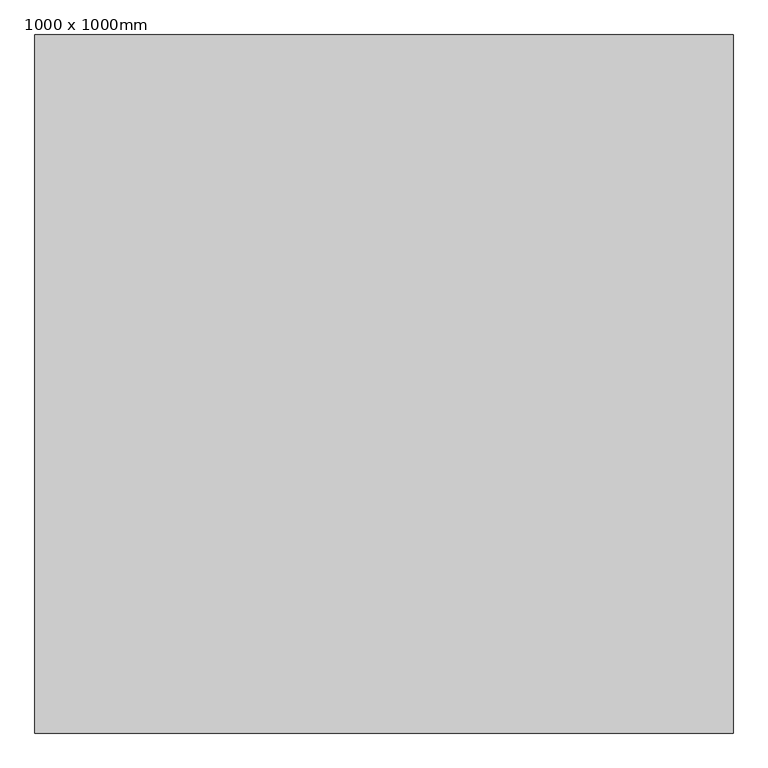
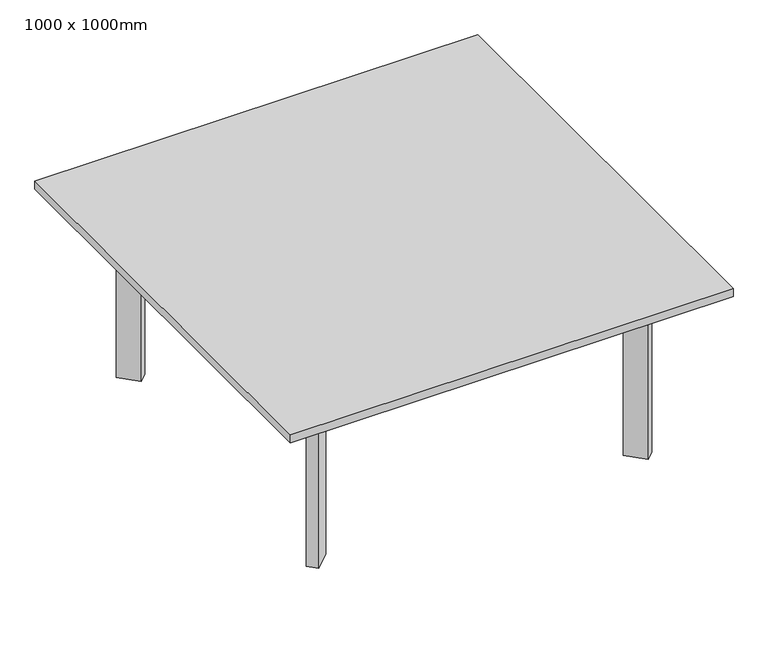
"""IFC4 building model written with IfcOpenShell, lengths in millimetres: furniture geometry, 1000 x 1000mm."""

from ifc_helpers import new_model, si_unit, frame, origin, origin_with_axes, place, context, project, spatial, polyline, outline, extrude, source, transform, mapped, element, save


def furniture_1000_x_1000mm_85c88e14(model_context):
    return source(origin(), model_context, "Body", "SweptSolid", [
        extrude(outline(polyline([(444.6325628, 440.0522349), (444.6325628, -559.9735464), (-555.3932185, -559.9735464), (-555.3932185, 440.0522349), (444.6325628, 440.0522349)])), frame((0.0, 0.0, 410.9640625), z_axis=(0.0, 0.0, 1.0), x_axis=(1.0, 0.0, 0.0)), (0.0, 0.0, 1.0), 19.05),
        extrude(outline(polyline([(-427.4000717, 330.0196004), (-391.4790473, 294.0985759), (-409.4395595, 276.1380637), (-445.360584, 312.0590881), (-427.4000717, 330.0196004)])), origin_with_axes(), (0.0, 0.0, 1.0), 360.1640625),
        extrude(outline(polyline([(316.639416, 330.0196004), (334.5999283, 312.0590881), (298.6789038, 276.1380637), (280.7183915, 294.0985759), (316.639416, 330.0196004)])), origin_with_axes(), (0.0, 0.0, 1.0), 360.1640625),
        extrude(outline(polyline([(334.5999283, -431.9803996), (316.639416, -449.9409119), (280.7183915, -414.0198874), (298.6789038, -396.0593751), (334.5999283, -431.9803996)])), origin_with_axes(), (0.0, 0.0, 1.0), 360.1640625),
        extrude(outline(polyline([(-445.360584, -431.9803996), (-409.4395595, -396.0593751), (-391.4790473, -414.0198874), (-427.4000717, -449.9409119), (-445.360584, -431.9803996)])), origin_with_axes(), (0.0, 0.0, 1.0), 360.1640625),
        extrude(outline(polyline([(-427.4000717, 330.0196004), (-55.3803279, -42.0001435), (316.639416, 330.0196004), (334.5999283, 312.0590881), (-37.4198156, -59.9606557), (334.5999283, -431.9803996), (316.639416, -449.9409119), (-55.3803279, -77.921168), (-427.4000717, -449.9409119), (-445.360584, -431.9803996), (-73.3408401, -59.9606557), (-445.360584, 312.0590881), (-427.4000717, 330.0196004)])), frame((0.0, 0.0, 360.1640625), z_axis=(0.0, 0.0, 1.0), x_axis=(1.0, 0.0, 0.0)), (0.0, 0.0, 1.0), 50.8),
    ])


if __name__ == "__main__":
    model = new_model("IFC4")
    model_context = context("Model", 3, world=origin())
    ifc_project = project(units=[si_unit("LENGTHUNIT", "METRE", prefix="MILLI")], contexts=[model_context])
    site = spatial("IfcSite", under=ifc_project)
    building = spatial("IfcBuilding", under=site)
    placement = place(None, origin())
    furniture_1000_x_1000mm_shape = furniture_1000_x_1000mm_85c88e14(model_context)
    element("IfcFurniture", 1, ObjectType="1000 x 1000mm", at=placement, inside=building, context=model_context, shape_type="MappedRepresentation", body=[
        mapped(furniture_1000_x_1000mm_shape, transform((0.0, 0.0, 0.0), x_axis=(1.0, 0.0, 0.0), y_axis=(0.0, 1.0, 0.0), z_axis=(0.0, 0.0, 1.0))),
    ])
    save(model, "model.ifc")

# Revit data of these elements
# Type "1000 x 1000mm"
#   Height = 1' - 4 119/128"
#   Length = 3' - 3 95/256"
#   Width = 3' - 3 95/256"
#   Default Elevation = 0
#   Assembly Code = ""
# Element 1 (IfcFurniture, "1000 x 1000mm")
#   Materials on its faces: "Metal - Steel, Polished", "Glass - Clear, Grey"
# Materials
#   "Metal - Steel, Polished": colour RGB 57 57 57, transparency 0
#   "Glass - Clear, Grey": colour RGB 252 255 255, transparency 0.64
